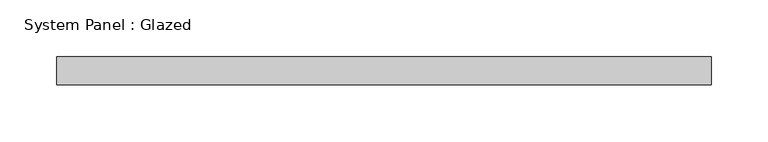
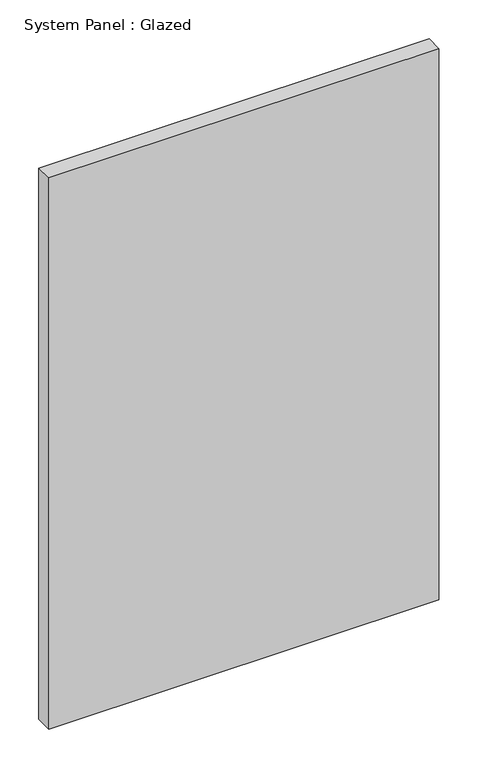
"""IFC4 building model written with IfcOpenShell, lengths in millimetres: plate geometry, System Panel : Glazed."""

from ifc_helpers import new_model, si_unit, origin, origin_with_axes, place, context, project, spatial, polyline, outline, extrude, source, transform, mapped, element, save


def system_panel_glazed_d3aa7d51(model_context):
    return source(origin(), model_context, "Body", "SweptSolid", [
        extrude(outline(polyline([(289.325, 24.5), (-289.325, 24.5), (-289.325, 49.5), (289.325, 49.5), (289.325, 24.5)])), origin_with_axes(), (0.0, 0.0, 1.0), 864.4),
    ])


if __name__ == "__main__":
    model = new_model("IFC4")
    model_context = context("Model", 3, world=origin())
    ifc_project = project(units=[si_unit("LENGTHUNIT", "METRE", prefix="MILLI")], contexts=[model_context])
    site = spatial("IfcSite", under=ifc_project)
    building = spatial("IfcBuilding", under=site)
    placement = place(None, origin())
    system_panel_glazed_shape = system_panel_glazed_d3aa7d51(model_context)
    element("IfcPlate", 1, ObjectType="System Panel : Glazed", at=placement, inside=building, context=model_context, shape_type="MappedRepresentation", body=[
        mapped(system_panel_glazed_shape, transform((0.0, 0.0, 0.0), x_axis=(1.0, 0.0, 0.0), y_axis=(0.0, 1.0, 0.0), z_axis=(0.0, 0.0, 1.0))),
    ])
    save(model, "model.ifc")

# Revit data of these elements
# Type "System Panel : Glazed"
#   Keynote = "H11"
#   Construction Type Id = "GSP4R"
#   Analytic Construction = "1/8 in Pilkington single glazing"
#   Visual Light Transmittance = 0.9
#   Solar Heat Gain Coefficient = 0.86
#   Heat Transfer Coefficient (U) = 6.7069 W/(m²·K)
#   Define Thermal Properties by = 1
# Element 1 (IfcPlate, "System Panel : Glazed")
#   Materials on its faces: "Glass"
# Materials
#   "Glass": class "Glass", colour RGB 0 128 192, transparency 0.9, Description = "Soda Lime Glass", Cost = 0
